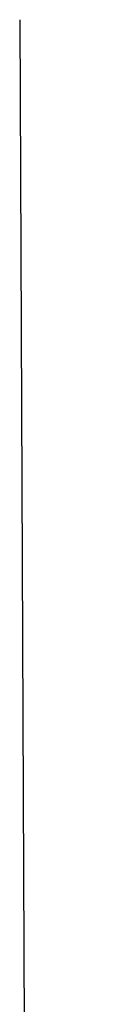
# Model space of a CAD drawing. Units: millimetres. Extents: x 1605 to 2079, y 1280 to 1879.
# Tile 7 of 7: x 1783 to 1812, y 1589 to 1879. Entities that reach past the tile are written whole.
import ezdxf

# ---------------------------------------------------------------- set-up
doc = ezdxf.new("R2010")
doc.units = ezdxf.units.MM
doc.layers.add('M-DIMS', color=2, linetype='Continuous', lineweight=25)
doc.styles.get("Standard").update_dxf_attribs({"font": 'arial.ttf'})
doc.dimstyles.new('ISO-25', dxfattribs={"dimtxt": 2.5, "dimasz": 2.5, "dimexe": 1.25, "dimexo": 0.625, "dimtad": 1, "dimdec": 0, "dimtxsty": 'Standard', "dimcen": 2.5, "dimadec": 0, "dimazin": 0, "dimtfac": 1, "dimtdec": 0, "dimtmove": 0, "dimatfit": 3, "dimfxl": 1, "dimarcsym": 0})

# ---------------------------------------------------------------- blocks, each defined once
blk = doc.blocks.new('*D17')
at = {"layer": 'Defpoints', "color": 0, "transparency": 16777216}
for p in [(1783.42, 1878.81), (1811.14, 1509.27)]:
    blk.add_point(p, dxfattribs=at)
at = {"layer": 'M-DIMS', "color": 0, "lineweight": -2, "transparency": 16777216}
blk.add_line((1808.13, 1549.43), (1810.96, 1511.76), dxfattribs=at)
at = {"layer": 'M-DIMS', "color": 0, "transparency": 16777216}
blk.add_solid([(1811.37, 1511.8), (1810.54, 1511.73), (1811.14, 1509.27)], dxfattribs=at)
at = {"layer": 'M-DIMS', "color": 0, "transparency": 16777216, "insert": (1810.35, 1545.24), "char_height": 2.5, "attachment_point": 5, "rotation": 274.2909}
blk.add_mtext('R371', dxfattribs=at)
blk = doc.blocks.new('*D71')
at = {"layer": 'Defpoints', "color": 0, "transparency": 16777216}
for p in [(1783.42, 1878.81), (1785.02, 1508.24)]:
    blk.add_point(p, dxfattribs=at)
at = {"layer": 'M-DIMS', "color": 0, "lineweight": -2, "transparency": 16777216}
for p, q in [((1783.42, 1878.81), (1785.02, 1508.24)), ((1786.01, 1279.86), (1785.03, 1505.74))]:
    blk.add_line(p, q, dxfattribs=at)
at = {"layer": 'M-DIMS', "color": 0, "transparency": 16777216}
blk.add_solid([(1785.45, 1505.74), (1784.61, 1505.73), (1785.02, 1508.24)], dxfattribs=at)
at = {"layer": 'M-DIMS', "color": 0, "transparency": 16777216, "insert": (1787.88, 1285.9), "char_height": 2.5, "attachment_point": 5, "rotation": 270.2478}
blk.add_mtext('R370.6', dxfattribs=at)

msp = doc.modelspace()

# ---------------------------------------------------------------- dimensions: what is measured, and where the dimension line sits
at = {"layer": 'M-DIMS'}
for mpoint, override, picture, middle in [((1811.1421, 1509.2717), {"dimclrd": 0, "dimclre": 0, "dimclrt": 0}, '*D17', (1808.4541, 1545.0966)), ((1785.0189, 1508.2365), {"dimdec": 1, "dimlfac": 1, "dimrnd": 0, "dimzin": 0, "dimdsep": 46, "dimlunit": 2}, '*D71', (1785.9807, 1285.8942))]:
    dim = msp.add_radius_dim(center=(1783.4159, 1878.8069), mpoint=mpoint, dimstyle='ISO-25', override=override, dxfattribs=at)
    dim.commit()
    dim.dimension.update_dxf_attribs({"geometry": picture, "text_midpoint": middle, "dimtype": 164})

doc.saveas('drawing.dxf')
